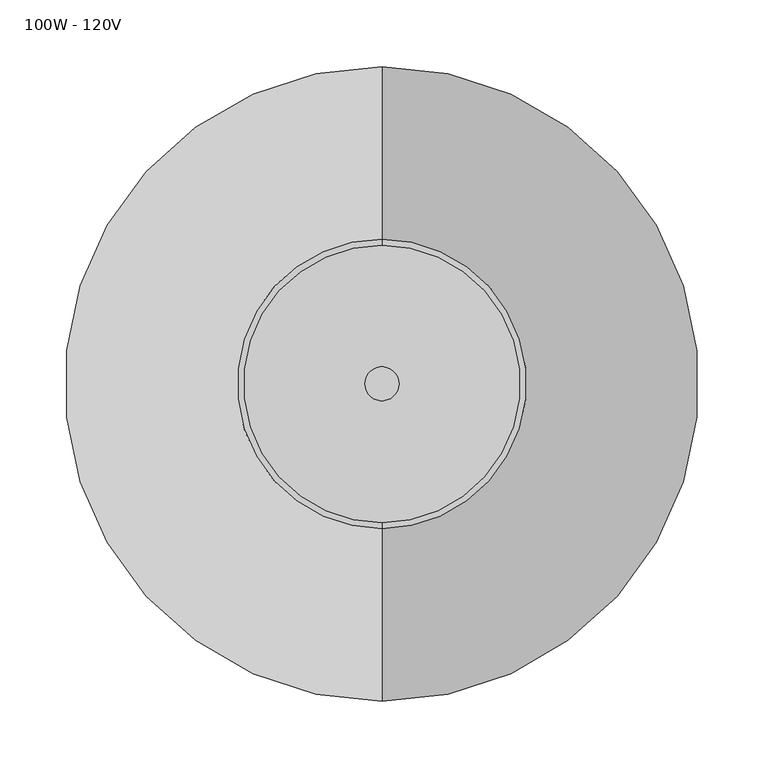
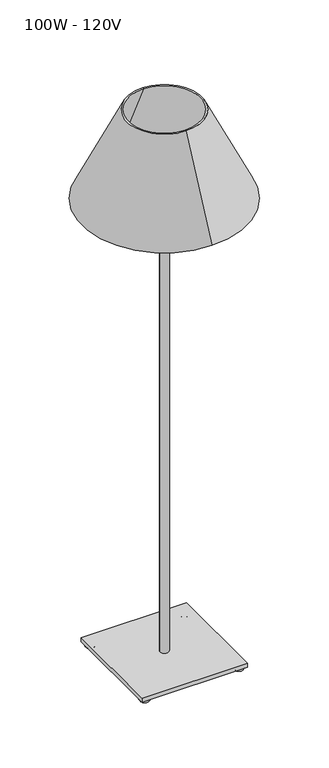
"""IFC4 building model written with IfcOpenShell, lengths in millimetres: light fixture geometry, 100W - 120V."""

from ifc_helpers import new_model, si_unit, point, frame, origin, origin_2d, place, context, project, spatial, polyline, circle_curve, ellipse_curve, trimmed, segment, composite_curve, outline, extrude, source, transform, mapped, element, save
from ifc_brep_helpers import plane_surface, revolved_surface, advanced_brep


def light_fixture_100w_120v_8564026f(model_context):
    return source(origin(), model_context, "Body", "SolidModel", [
        extrude(outline(composite_curve([segment(trimmed(circle_curve(origin_2d(), 12.7), [point((-12.7, 0.0))], [point((12.7, 0.0))], False, "CARTESIAN"), True, "CONTINUOUS"), segment(trimmed(circle_curve(origin_2d(), 12.7), [point((12.7, 0.0))], [point((-12.7, 0.0))], False, "CARTESIAN"), True, "CONTINUOUS")], self_intersect=False)), frame((0.0, 0.0, 24.9639672), z_axis=(0.0, 0.0, 1.0), x_axis=(1.0, 0.0, 0.0)), (0.0, 0.0, 1.0), 1499.0360328),
        extrude(outline(polyline([(152.4, 152.4), (152.4, -152.4), (-152.4, -152.4), (-152.4, 152.4), (152.4, 152.4)])), frame((0.0, 0.0, 12.6871384), z_axis=(0.0, 0.0, 1.0), x_axis=(1.0, 0.0, 0.0)), (0.0, 0.0, 1.0), 12.2768288),
        advanced_brep(
        [(133.9366871, -135.595774, 0.0), (140.1544999, -135.595774, 0.0), (140.1544999, -135.595774, 12.6871384), (133.9366871, -135.595774, 12.6871384), (121.2495488, -135.595774, 12.6871384), (152.8416383, -135.595774, 12.6871384)],
        [
            (0, 1, circle_curve(frame((137.0455935, -135.595774, 0.0), z_axis=(0.0, 0.0, -1.0), x_axis=(0.0, 1.0, 0.0)), 3.1089064)),
            (1, 2),
            (2, 3, circle_curve(frame((137.0455935, -135.595774, 12.6871384), z_axis=(0.0, 0.0, 1.0), x_axis=(0.0, 1.0, 0.0)), 3.1089064)),
            (3, 0),
            (1, 0, circle_curve(frame((137.0455935, -135.595774, 0.0), z_axis=(0.0, 0.0, -1.0), x_axis=(0.0, 1.0, 0.0)), 3.1089064)),
            (3, 2, circle_curve(frame((137.0455935, -135.595774, 12.6871384), z_axis=(0.0, 0.0, 1.0), x_axis=(0.0, 1.0, 0.0)), 3.1089064)),
            (4, 5, circle_curve(frame((137.0455935, -135.595774, 12.6871384), z_axis=(0.0, 0.0, -1.0), x_axis=(0.0, 1.0, 0.0)), 15.7960447)),
            (5, 1, circle_curve(frame((140.1544999, -135.595774, 12.6871384), z_axis=(0.0, 1.0, 0.0), x_axis=(1.0, 0.0, 0.0)), 12.6871384)),
            (0, 4, circle_curve(frame((133.9366871, -135.595774, 12.6871384), z_axis=(0.0, 1.0, 0.0), x_axis=(-1.0, 0.0, 0.0)), 12.6871384)),
            (5, 4, circle_curve(frame((137.0455935, -135.595774, 12.6871384), z_axis=(0.0, 0.0, -1.0), x_axis=(0.0, 1.0, 0.0)), 15.7960447)),
            (2, 5),
            (4, 3),
        ],
        [
            revolved_surface(polyline([(137.0455935, -132.4868676, 12.6871384), (137.0455935, -132.4868676, 0.0)]), (137.0455935, -135.595774, 0.0), (0.0, 0.0, 1.0)),
            revolved_surface(trimmed(ellipse_curve(frame((137.0455935, -132.4868676, 12.6871384), z_axis=(1.0, 0.0, 0.0), x_axis=(0.0, 1.0, 0.0)), 12.6871384, 12.6871384), [point((137.0455935, -132.4868676, 0.0))], [point((137.0455935, -119.7997292, 12.6871384))], True, "CARTESIAN"), (137.0455935, -135.595774, 0.0), (0.0, 0.0, 1.0)),
            plane_surface(frame((137.0455935, -135.595774, 12.6871384), z_axis=(0.0, 0.0, 1.0), x_axis=(0.0, 1.0, 0.0))),
        ],
        [
            (0, [[1, 2, 3, 4]]),
            (0, [[5, -4, 6, -2]]),
            (1, [[7, 8, -1, 9]]),
            (1, [[10, -9, -5, -8]]),
            (2, [[-3, 11, -7, 12]]),
            (2, [[-6, -12, -10, -11]]),
        ],
    ),
        advanced_brep(
        [(-138.5460372, -136.1907144, 0.0), (-132.3282244, -136.1907144, 0.0), (-132.3282244, -136.1907144, 12.6871384), (-138.5460372, -136.1907144, 12.6871384), (-151.2331755, -136.1907144, 12.6871384), (-119.641086, -136.1907144, 12.6871384)],
        [
            (0, 1, circle_curve(frame((-135.4371308, -136.1907144, 0.0), z_axis=(0.0, 0.0, -1.0), x_axis=(0.0, 1.0, 0.0)), 3.1089064)),
            (1, 2),
            (2, 3, circle_curve(frame((-135.4371308, -136.1907144, 12.6871384), z_axis=(0.0, 0.0, 1.0), x_axis=(0.0, 1.0, 0.0)), 3.1089064)),
            (3, 0),
            (1, 0, circle_curve(frame((-135.4371308, -136.1907144, 0.0), z_axis=(0.0, 0.0, -1.0), x_axis=(0.0, 1.0, 0.0)), 3.1089064)),
            (3, 2, circle_curve(frame((-135.4371308, -136.1907144, 12.6871384), z_axis=(0.0, 0.0, 1.0), x_axis=(0.0, 1.0, 0.0)), 3.1089064)),
            (4, 5, circle_curve(frame((-135.4371308, -136.1907144, 12.6871384), z_axis=(0.0, 0.0, -1.0), x_axis=(0.0, 1.0, 0.0)), 15.7960447)),
            (5, 1, circle_curve(frame((-132.3282244, -136.1907144, 12.6871384), z_axis=(0.0, 1.0, 0.0), x_axis=(1.0, 0.0, 0.0)), 12.6871384)),
            (0, 4, circle_curve(frame((-138.5460372, -136.1907144, 12.6871384), z_axis=(0.0, 1.0, 0.0), x_axis=(-1.0, 0.0, 0.0)), 12.6871384)),
            (5, 4, circle_curve(frame((-135.4371308, -136.1907144, 12.6871384), z_axis=(0.0, 0.0, -1.0), x_axis=(0.0, 1.0, 0.0)), 15.7960447)),
            (2, 5),
            (4, 3),
        ],
        [
            revolved_surface(polyline([(-135.4371308, -133.081808, 12.6871384), (-135.4371308, -133.081808, 0.0)]), (-135.4371308, -136.1907144, 0.0), (0.0, 0.0, 1.0)),
            revolved_surface(trimmed(ellipse_curve(frame((-135.4371308, -133.081808, 12.6871384), z_axis=(1.0, 0.0, 0.0), x_axis=(0.0, 1.0, 0.0)), 12.6871384, 12.6871384), [point((-135.4371308, -133.081808, 0.0))], [point((-135.4371308, -120.3946697, 12.6871384))], True, "CARTESIAN"), (-135.4371308, -136.1907144, 0.0), (0.0, 0.0, 1.0)),
            plane_surface(frame((-135.4371308, -136.1907144, 12.6871384), z_axis=(0.0, 0.0, 1.0), x_axis=(0.0, 1.0, 0.0))),
        ],
        [
            (0, [[1, 2, 3, 4]]),
            (0, [[5, -4, 6, -2]]),
            (1, [[7, 8, -1, 9]]),
            (1, [[10, -9, -5, -8]]),
            (2, [[-3, 11, -7, 12]]),
            (2, [[-6, -12, -10, -11]]),
        ],
    ),
        advanced_brep(
        [(-139.1409776, 135.6970694, 0.0), (-132.9231648, 135.6970694, 0.0), (-132.9231648, 135.6970694, 12.6871384), (-139.1409776, 135.6970694, 12.6871384), (-151.828116, 135.6970694, 12.6871384), (-120.2360265, 135.6970694, 12.6871384)],
        [
            (0, 1, circle_curve(frame((-136.0320712, 135.6970694, 0.0), z_axis=(0.0, 0.0, -1.0), x_axis=(0.0, 1.0, 0.0)), 3.1089064)),
            (1, 2),
            (2, 3, circle_curve(frame((-136.0320712, 135.6970694, 12.6871384), z_axis=(0.0, 0.0, 1.0), x_axis=(0.0, 1.0, 0.0)), 3.1089064)),
            (3, 0),
            (1, 0, circle_curve(frame((-136.0320712, 135.6970694, 0.0), z_axis=(0.0, 0.0, -1.0), x_axis=(0.0, 1.0, 0.0)), 3.1089064)),
            (3, 2, circle_curve(frame((-136.0320712, 135.6970694, 12.6871384), z_axis=(0.0, 0.0, 1.0), x_axis=(0.0, 1.0, 0.0)), 3.1089064)),
            (4, 5, circle_curve(frame((-136.0320712, 135.6970694, 12.6871384), z_axis=(0.0, 0.0, -1.0), x_axis=(0.0, 1.0, 0.0)), 15.7960447)),
            (5, 1, circle_curve(frame((-132.9231648, 135.6970694, 12.6871384), z_axis=(0.0, 1.0, 0.0), x_axis=(1.0, 0.0, 0.0)), 12.6871384)),
            (0, 4, circle_curve(frame((-139.1409776, 135.6970694, 12.6871384), z_axis=(0.0, 1.0, 0.0), x_axis=(-1.0, 0.0, 0.0)), 12.6871384)),
            (5, 4, circle_curve(frame((-136.0320712, 135.6970694, 12.6871384), z_axis=(0.0, 0.0, -1.0), x_axis=(0.0, 1.0, 0.0)), 15.7960447)),
            (2, 5),
            (4, 3),
        ],
        [
            revolved_surface(polyline([(-136.0320712, 138.8059758, 12.6871384), (-136.0320712, 138.8059758, 0.0)]), (-136.0320712, 135.6970694, 0.0), (0.0, 0.0, 1.0)),
            revolved_surface(trimmed(ellipse_curve(frame((-136.0320712, 138.8059758, 12.6871384), z_axis=(1.0, 0.0, 0.0), x_axis=(0.0, 1.0, 0.0)), 12.6871384, 12.6871384), [point((-136.0320712, 138.8059758, 0.0))], [point((-136.0320712, 151.4931142, 12.6871384))], True, "CARTESIAN"), (-136.0320712, 135.6970694, 0.0), (0.0, 0.0, 1.0)),
            plane_surface(frame((-136.0320712, 135.6970694, 12.6871384), z_axis=(0.0, 0.0, 1.0), x_axis=(0.0, 1.0, 0.0))),
        ],
        [
            (0, [[1, 2, 3, 4]]),
            (0, [[5, -4, 6, -2]]),
            (1, [[7, 8, -1, 9]]),
            (1, [[10, -9, -5, -8]]),
            (2, [[-3, 11, -7, 12]]),
            (2, [[-6, -12, -10, -11]]),
        ],
    ),
        advanced_brep(
        [(133.2106985, 136.0573029, 0.0), (139.4285113, 136.0573029, 0.0), (139.4285113, 136.0573029, 12.6871384), (133.2106985, 136.0573029, 12.6871384), (120.5235602, 136.0573029, 12.6871384), (152.1156497, 136.0573029, 12.6871384)],
        [
            (0, 1, circle_curve(frame((136.3196049, 136.0573029, 0.0), z_axis=(0.0, 0.0, -1.0), x_axis=(0.0, 1.0, 0.0)), 3.1089064)),
            (1, 2),
            (2, 3, circle_curve(frame((136.3196049, 136.0573029, 12.6871384), z_axis=(0.0, 0.0, 1.0), x_axis=(0.0, 1.0, 0.0)), 3.1089064)),
            (3, 0),
            (1, 0, circle_curve(frame((136.3196049, 136.0573029, 0.0), z_axis=(0.0, 0.0, -1.0), x_axis=(0.0, 1.0, 0.0)), 3.1089064)),
            (3, 2, circle_curve(frame((136.3196049, 136.0573029, 12.6871384), z_axis=(0.0, 0.0, 1.0), x_axis=(0.0, 1.0, 0.0)), 3.1089064)),
            (4, 5, circle_curve(frame((136.3196049, 136.0573029, 12.6871384), z_axis=(0.0, 0.0, -1.0), x_axis=(0.0, 1.0, 0.0)), 15.7960447)),
            (5, 1, circle_curve(frame((139.4285113, 136.0573029, 12.6871384), z_axis=(0.0, 1.0, 0.0), x_axis=(1.0, 0.0, 0.0)), 12.6871384)),
            (0, 4, circle_curve(frame((133.2106985, 136.0573029, 12.6871384), z_axis=(0.0, 1.0, 0.0), x_axis=(-1.0, 0.0, 0.0)), 12.6871384)),
            (5, 4, circle_curve(frame((136.3196049, 136.0573029, 12.6871384), z_axis=(0.0, 0.0, -1.0), x_axis=(0.0, 1.0, 0.0)), 15.7960447)),
            (2, 5),
            (4, 3),
        ],
        [
            revolved_surface(polyline([(136.3196049, 139.1662093, 12.6871384), (136.3196049, 139.1662093, 0.0)]), (136.3196049, 136.0573029, 0.0), (0.0, 0.0, 1.0)),
            revolved_surface(trimmed(ellipse_curve(frame((136.3196049, 139.1662093, 12.6871384), z_axis=(1.0, 0.0, 0.0), x_axis=(0.0, 1.0, 0.0)), 12.6871384, 12.6871384), [point((136.3196049, 139.1662093, 0.0))], [point((136.3196049, 151.8533477, 12.6871384))], True, "CARTESIAN"), (136.3196049, 136.0573029, 0.0), (0.0, 0.0, 1.0)),
            plane_surface(frame((136.3196049, 136.0573029, 12.6871384), z_axis=(0.0, 0.0, 1.0), x_axis=(0.0, 1.0, 0.0))),
        ],
        [
            (0, [[1, 2, 3, 4]]),
            (0, [[5, -4, 6, -2]]),
            (1, [[7, 8, -1, 9]]),
            (1, [[10, -9, -5, -8]]),
            (2, [[-3, 11, -7, 12]]),
            (2, [[-6, -12, -10, -11]]),
        ],
    ),
        advanced_brep(
        [(0.0, -233.3382251, 1403.5752564), (0.0, 233.3382251, 1403.5752564), (0.0, 104.0586089, 1674.1859784), (0.0, -104.0586089, 1674.1859784), (0.0, -237.8523754, 1403.5752564), (0.0, 237.8523754, 1403.5752564), (0.0, -108.5727592, 1674.1859784), (0.0, 108.5727592, 1674.1859784)],
        [
            (0, 1, circle_curve(frame((0.0, 0.0, 1403.5752564), z_axis=(0.0, 0.0, -1.0), x_axis=(0.0, 1.0, 0.0)), 233.3382251)),
            (1, 2),
            (2, 3, circle_curve(frame((0.0, 0.0, 1674.1859784), z_axis=(0.0, 0.0, 1.0), x_axis=(0.0, 1.0, 0.0)), 104.0586089)),
            (3, 0),
            (1, 0, circle_curve(frame((0.0, 0.0, 1403.5752564), z_axis=(0.0, 0.0, -1.0), x_axis=(0.0, 1.0, 0.0)), 233.3382251)),
            (3, 2, circle_curve(frame((0.0, 0.0, 1674.1859784), z_axis=(0.0, 0.0, 1.0), x_axis=(0.0, 1.0, 0.0)), 104.0586089)),
            (4, 5, circle_curve(frame((0.0, 0.0, 1403.5752564), z_axis=(0.0, 0.0, -1.0), x_axis=(0.0, 1.0, 0.0)), 237.8523754)),
            (5, 1),
            (0, 4),
            (5, 4, circle_curve(frame((0.0, 0.0, 1403.5752564), z_axis=(0.0, 0.0, -1.0), x_axis=(0.0, 1.0, 0.0)), 237.8523754)),
            (6, 7, circle_curve(frame((0.0, 0.0, 1674.1859784), z_axis=(0.0, 0.0, -1.0), x_axis=(0.0, 1.0, 0.0)), 108.5727592)),
            (7, 5),
            (4, 6),
            (7, 6, circle_curve(frame((0.0, 0.0, 1674.1859784), z_axis=(0.0, 0.0, -1.0), x_axis=(0.0, 1.0, 0.0)), 108.5727592)),
            (2, 7),
            (6, 3),
        ],
        [
            revolved_surface(polyline([(0.0, 104.0586089, 1674.1859784), (0.0, 233.3382251, 1403.5752564)]), (0.0, 0.0, 1713.8233367), (0.0, 0.0, 1.0)),
            plane_surface(frame((0.0, 0.0, 1403.5752564), z_axis=(0.0, 0.0, -1.0), x_axis=(0.0, 1.0, 0.0))),
            revolved_surface(polyline([(0.0, 237.8523754, 1403.5752564), (0.0, 108.5727592, 1674.1859784)]), (0.0, 0.0, 1713.8233367), (0.0, 0.0, 1.0)),
            plane_surface(frame((0.0, 0.0, 1674.1859784), z_axis=(0.0, 0.0, 1.0), x_axis=(0.0, 1.0, 0.0))),
        ],
        [
            (0, [[1, 2, 3, 4]]),
            (0, [[5, -4, 6, -2]]),
            (1, [[7, 8, -1, 9]]),
            (1, [[10, -9, -5, -8]]),
            (2, [[11, 12, -7, 13]]),
            (2, [[14, -13, -10, -12]]),
            (3, [[-3, 15, -11, 16]]),
            (3, [[-6, -16, -14, -15]]),
        ],
    ),
    ])


if __name__ == "__main__":
    model = new_model("IFC4")
    model_context = context("Model", 3, world=origin())
    ifc_project = project(units=[si_unit("LENGTHUNIT", "METRE", prefix="MILLI")], contexts=[model_context])
    site = spatial("IfcSite", under=ifc_project)
    building = spatial("IfcBuilding", under=site)
    placement = place(None, origin())
    light_fixture_100w_120v_shape = light_fixture_100w_120v_8564026f(model_context)
    element("IfcLightFixture", 1, ObjectType="100W - 120V", at=placement, inside=building, context=model_context, shape_type="MappedRepresentation", body=[
        mapped(light_fixture_100w_120v_shape, transform((0.0, 0.0, 0.0), x_axis=(1.0, 0.0, 0.0), y_axis=(0.0, 1.0, 0.0), z_axis=(0.0, 0.0, 1.0))),
    ])
    save(model, "model.ifc")

# Revit data of these elements
# Type "100W - 120V"
#   Assembly Code = "D5020220"
#   Lamp = "A-19"
#   Wattage Comments = "100"
#   Wattage = 100 W
#   built-in parameter 1150110 = 1 (stored number, unit not read)
#   built-in parameter 1114217 = 1 (stored number, unit not read)
#   built-in parameter 1150109 = 1 (stored number, unit not read)
#   built-in parameter 1150113 = 1 (stored number, unit not read)
#   built-in parameter 1150115 = 1 (stored number, unit not read)
#   built-in parameter 1150105 = 139.261 (stored number, unit not read)
#   Light Source Symbol Size = 2' - 0"
#   built-in parameter 1150112 = 1 (stored number, unit not read)
#   built-in parameter 1150114 = 1 (stored number, unit not read)
#   built-in parameter 1150107 = 2800 (stored number, unit not read)
#   built-in parameter 1150106 = 1.39261 (stored number, unit not read)
#   built-in parameter 1150104 = 1.6258 (stored number, unit not read)
#   Ballast Voltage = 120 V
#   built-in parameter 1114218 = 1 (stored number, unit not read)
#   built-in parameter 1150133 = 10 (stored number, unit not read)
#   Lumens = 1750 lm
#   Apparent Load = 100 VA
#   built-in parameter 1150134 = 4
#   built-in parameter 1150137 = 1
#   Color Filter = 16777215
#   Ballast Number of Poles = 1
#   Shade = Glass, Frosted
#   Stand = Steel, Chrome Plated
#   Dimming Lamp Color Temperature Shift = (empty or 0)
#   Default Elevation = 0
# Element 1 (IfcLightFixture, "100W - 120V")
#   Materials on its faces: "Steel, Chrome Plated", "Glass, Frosted"
# Materials
#   "Glass, Frosted": class "Glass", colour RGB 250 244 225, transparency 0.55, Description = "physical material", Cost = 0
#   "Steel, Chrome Plated": class "Metal", colour RGB 17 17 17, transparency 0, Description = "Chromiuim plated steel", Cost = 0
